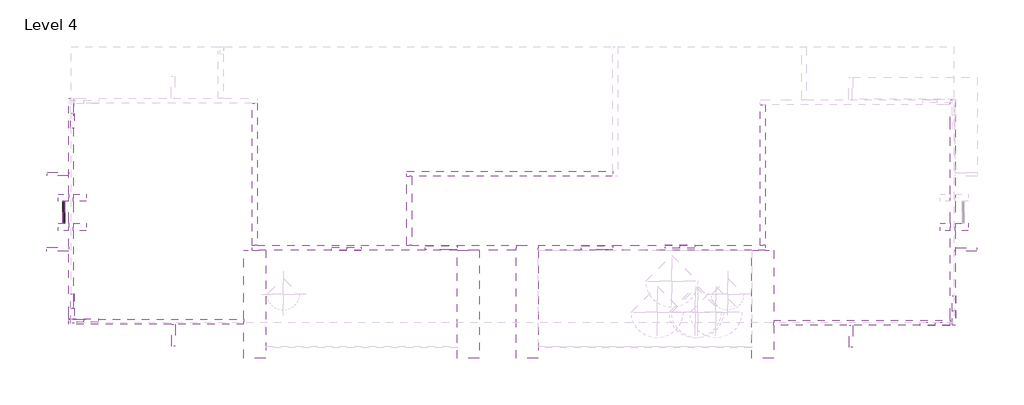
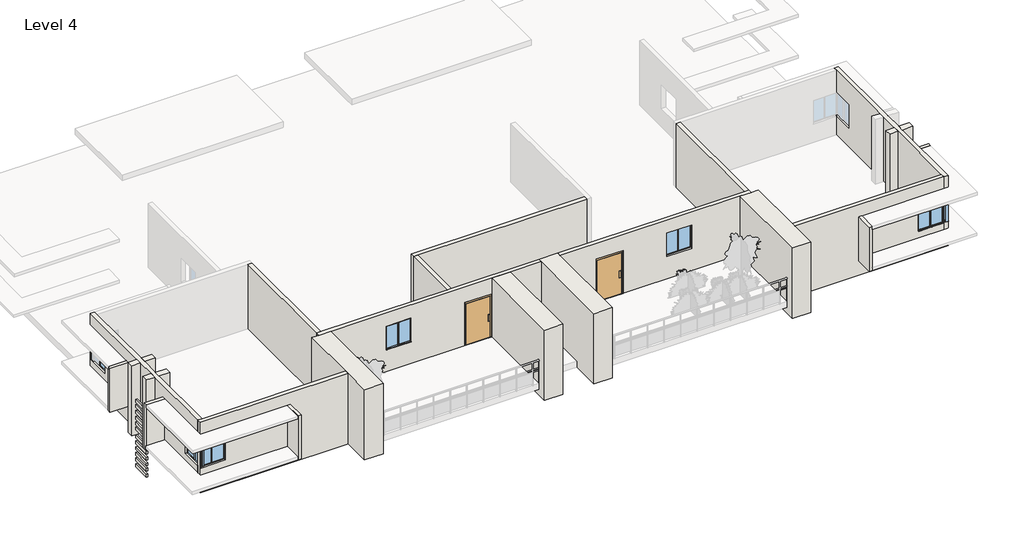
# One storey, part 1 of 4: 49 walls, 13 windows, 2 doors.
"""IFC4 building model written with IfcOpenShell, lengths in millimetres."""

from ifc_helpers import new_model, si_unit, frame, origin, place, context, project, spatial, polyline, outline, extrude, faceted_brep, transform, mapped, element, save
from components import door_15d3c954, window_20ff4747

model = new_model("IFC4")

# Units and contexts
model_context = context("Model", 3, world=origin())
ifc_project = project(units=[si_unit("LENGTHUNIT", "METRE", prefix="MILLI")], contexts=[model_context])

# Site, building, storey
site = spatial("IfcSite", under=ifc_project)
building = spatial("IfcBuilding", under=site)
storey = spatial("IfcBuildingStorey", under=building, Name="Level 4", Elevation=9144.0)

# Doors
placement = place(None, origin())
door_shape = door_15d3c954(model_context)
element("IfcDoor", 1, ObjectType="Door-Passage-Single-Flush-Dbl_Acting : 48\" x 96\"", at=placement, inside=storey, context=model_context, shape_type="MappedRepresentation", body=[
    mapped(door_shape, transform((7011.0520665, -5255.880811, 10972.8), x_axis=(-1.0, 0.0, 0.0), y_axis=(0.0, -1.0, 0.0), z_axis=(0.0, 0.0, 1.0))),
])
element("IfcDoor", 2, ObjectType="Door-Passage-Single-Flush-Dbl_Acting : 48\" x 96\"", at=placement, inside=storey, context=model_context, shape_type="MappedRepresentation", body=[
    mapped(door_shape, transform((559.4520665, -5255.1961695, 10972.8), x_axis=(-1.0, 0.0, 0.0), y_axis=(0.0, -1.0, 0.0), z_axis=(0.0, 0.0, 1.0))),
])

# Walls
element("IfcWall", 3, ObjectType="Generic - 1'", at=placement, inside=storey, context=model_context, shape_type="SweptSolid", body=[
    extrude(outline(polyline([(-14151.7972154, -3343.5294056), (-14680.5479335, -3343.5294056), (-14680.5479335, -3038.7294056), (-14151.7972154, -3038.7294056), (-14151.7972154, -3343.5294056)])), frame((0.0, 0.0, 10363.2), z_axis=(0.0, 0.0, 1.0), x_axis=(1.0, 0.0, 0.0)), (0.0, 0.0, 1.0), 3657.6),
])
element("IfcWall", 4, ObjectType="Generic - 1'", at=placement, inside=storey, context=model_context, shape_type="SweptSolid", body=[
    extrude(outline(polyline([(-15302.1394029, -3038.7294056), (-14883.7479335, -3038.7294056), (-14883.7479335, -3343.5294056), (-15302.1394029, -3343.5294056), (-15302.1394029, -3038.7294056)])), frame((0.0, 0.0, 10363.2), z_axis=(0.0, 0.0, 1.0), x_axis=(1.0, 0.0, 0.0)), (0.0, 0.0, 1.0), 3657.6),
])
element("IfcWall", 5, ObjectType="Generic - 1'", at=placement, inside=storey, context=model_context, shape_type="SweptSolid", body=[
    extrude(outline(polyline([(-14151.7972154, -4562.7294056), (-14680.5479335, -4562.7294056), (-14680.5479335, -4257.9294056), (-14151.7972154, -4257.9294056), (-14151.7972154, -4562.7294056)])), frame((0.0, 0.0, 10363.2), z_axis=(0.0, 0.0, 1.0), x_axis=(1.0, 0.0, 0.0)), (0.0, 0.0, 1.0), 3657.6),
])
element("IfcWall", 6, ObjectType="Generic - 1'", at=placement, inside=storey, context=model_context, shape_type="SweptSolid", body=[
    extrude(outline(polyline([(-15302.1394029, -4257.9294056), (-14883.7479335, -4257.9294056), (-14883.7479335, -4562.7294056), (-15302.1394029, -4562.7294056), (-15302.1394029, -4257.9294056)])), frame((0.0, 0.0, 10363.2), z_axis=(0.0, 0.0, 1.0), x_axis=(1.0, 0.0, 0.0)), (0.0, 0.0, 1.0), 3657.6),
])
element("IfcWall", 7, ObjectType="Generic - 1'", at=placement, inside=storey, context=model_context, shape_type="SweptSolid", body=[
    extrude(outline(polyline([(22386.1027846, -4562.7294056), (21857.3520665, -4562.7294056), (21857.3520665, -4257.9294056), (22386.1027846, -4257.9294056), (22386.1027846, -4562.7294056)])), frame((0.0, 0.0, 10363.2), z_axis=(0.0, 0.0, 1.0), x_axis=(1.0, 0.0, 0.0)), (0.0, 0.0, 1.0), 3657.6),
])
element("IfcWall", 8, ObjectType="Generic - 1'", at=placement, inside=storey, context=model_context, shape_type="SweptSolid", body=[
    extrude(outline(polyline([(21235.7605971, -4257.9294056), (21654.1520665, -4257.9294056), (21654.1520665, -4562.7294056), (21235.7605971, -4562.7294056), (21235.7605971, -4257.9294056)])), frame((0.0, 0.0, 10363.2), z_axis=(0.0, 0.0, 1.0), x_axis=(1.0, 0.0, 0.0)), (0.0, 0.0, 1.0), 3657.6),
])
element("IfcWall", 9, ObjectType="Generic - 3'", at=placement, inside=storey, context=model_context, shape_type="Brep", body=[
    faceted_brep([(2134.2520665, -9833.5461695, 10363.2), (2134.2520665, -5363.1461695, 10363.2), (2134.2520665, -5363.1461695, 14020.8), (2134.2520665, -9833.5461695, 14020.8), (1219.8520665, -9833.5461695, 10363.2), (1219.8520665, -9833.5461695, 14020.8), (1219.8520665, -5363.1461695, 14020.8), (1219.8520665, -5363.1461695, 13208.0), (1219.8520665, -5363.1461695, 10972.8), (1219.8520665, -5363.1461695, 10363.2)], [[[0, 1, 2, 3]], [[4, 5, 6, 7, 8, 9]], [[1, 0, 4, 9]], [[3, 2, 6, 5]], [[0, 3, 5, 4]], [[2, 1, 9, 8, 7, 6]]]),
])
element("IfcWall", 10, ObjectType="Generic - 3'", at=placement, inside=storey, context=model_context, shape_type="Brep", body=[
    faceted_brep([(4572.6520665, -9833.5461695, 10363.2), (4572.6520665, -5363.830811, 10363.2), (4572.6520665, -5160.630811, 10363.2), (4572.6520665, -5160.630811, 14020.8), (4572.6520665, -5363.830811, 14020.8), (4572.6520665, -9833.5461695, 14020.8), (3658.2520665, -9833.5461695, 10363.2), (3658.2520665, -9833.5461695, 14020.8), (3658.2520665, -5363.1461695, 14020.8), (3658.2520665, -5160.630811, 14020.8), (3658.2520665, -5160.630811, 10363.2), (3658.2520665, -5363.1461695, 10363.2)], [[[0, 1, 2, 3, 4, 5]], [[6, 7, 8, 9, 10, 11]], [[2, 1, 0, 6, 11, 10]], [[5, 4, 3, 9, 8, 7]], [[0, 5, 7, 6]], [[3, 2, 10, 9]]]),
])
element("IfcWall", 11, ObjectType="Generic - 3'", at=placement, inside=storey, context=model_context, shape_type="Brep", body=[
    faceted_brep([(-7619.3479335, -5363.1461695, 10363.2), (-7619.3479335, -8237.0604699, 10363.2), (-7619.3479335, -8440.2604699, 10363.2), (-7619.3479335, -9833.5461695, 10363.2), (-7619.3479335, -9833.5461695, 14020.8), (-7619.3479335, -8440.2604699, 14020.8), (-7619.3479335, -8237.0604699, 14020.8), (-7619.3479335, -5363.1461695, 14020.8), (-6704.9479335, -5363.1461695, 10363.2), (-6704.9479335, -5363.1461695, 14020.8), (-6704.9479335, -9833.5461695, 14020.8), (-6704.9479335, -9833.5461695, 10363.2), (-7263.7479335, -5363.1461695, 10363.2), (-7263.7479335, -5363.1461695, 14020.8)], [[[0, 1, 2, 3, 4, 5, 6, 7]], [[8, 9, 10, 11]], [[3, 2, 1, 0, 12, 8, 11]], [[4, 3, 11, 10]], [[7, 6, 5, 4, 10, 9, 13]], [[0, 7, 13, 9, 8, 12]]]),
])
element("IfcWall", 12, ObjectType="Generic - 3'", at=placement, inside=storey, context=model_context, shape_type="Brep", body=[
    faceted_brep([(13411.8520665, -5363.830811, 10363.2), (13411.8520665, -9834.230811, 10363.2), (13411.8520665, -9834.230811, 14020.8), (13411.8520665, -5363.830811, 14020.8), (14326.2520665, -5363.830811, 10363.2), (14326.2520665, -5363.830811, 14020.8), (14326.2520665, -8263.1451114, 14020.8), (14326.2520665, -8466.3451114, 14020.8), (14326.2520665, -9834.230811, 14020.8), (14326.2520665, -9834.230811, 10363.2), (14326.2520665, -8466.3451114, 10363.2), (14326.2520665, -8263.1451114, 10363.2), (13970.6520665, -5363.830811, 10363.2), (13970.6520665, -5363.830811, 14020.8)], [[[0, 1, 2, 3]], [[4, 5, 6, 7, 8, 9, 10, 11]], [[1, 0, 12, 4, 11, 10, 9]], [[2, 1, 9, 8]], [[3, 2, 8, 7, 6, 5, 13]], [[0, 3, 13, 5, 4, 12]]]),
])
element("IfcWall", 13, ObjectType="Generic - 5\"", at=placement, inside=storey, context=model_context, shape_type="SweptSolid", body=[
    extrude(outline(polyline([(-15124.6936682, -4257.9294056), (-15124.6936682, -3343.5294056), (-15048.4936682, -3343.5294056), (-15048.4936682, -4257.9294056), (-15124.6936682, -4257.9294056)])), frame((0.0, 0.0, 8712.2), z_axis=(0.0, 0.0, 1.0), x_axis=(1.0, 0.0, 0.0)), (0.0, 0.0, 1.0), 152.8735856),
])
element("IfcWall", 14, ObjectType="Generic - 5\"", at=placement, inside=storey, context=model_context, shape_type="SweptSolid", body=[
    extrude(outline(polyline([(-15124.6936682, -4257.9294056), (-15124.6936682, -3343.5294056), (-15048.4936682, -3343.5294056), (-15048.4936682, -4257.9294056), (-15124.6936682, -4257.9294056)])), frame((0.0, 0.0, 9017.0), z_axis=(0.0, 0.0, 1.0), x_axis=(1.0, 0.0, 0.0)), (0.0, 0.0, 1.0), 152.8735856),
])
element("IfcWall", 15, ObjectType="Generic - 5\"", at=placement, inside=storey, context=model_context, shape_type="SweptSolid", body=[
    extrude(outline(polyline([(-15124.6936682, -4257.9294056), (-15124.6936682, -3343.5294056), (-15048.4936682, -3343.5294056), (-15048.4936682, -4257.9294056), (-15124.6936682, -4257.9294056)])), frame((0.0, 0.0, 9296.4), z_axis=(0.0, 0.0, 1.0), x_axis=(1.0, 0.0, 0.0)), (0.0, 0.0, 1.0), 152.8735856),
])
element("IfcWall", 16, ObjectType="Generic - 5\"", at=placement, inside=storey, context=model_context, shape_type="SweptSolid", body=[
    extrude(outline(polyline([(-15124.6936682, -4257.9294056), (-15124.6936682, -3343.5294056), (-15048.4936682, -3343.5294056), (-15048.4936682, -4257.9294056), (-15124.6936682, -4257.9294056)])), frame((0.0, 0.0, 9601.2), z_axis=(0.0, 0.0, 1.0), x_axis=(1.0, 0.0, 0.0)), (0.0, 0.0, 1.0), 152.8735856),
])
element("IfcWall", 17, ObjectType="Generic - 5\"", at=placement, inside=storey, context=model_context, shape_type="SweptSolid", body=[
    extrude(outline(polyline([(-15124.6936682, -4257.9294056), (-15124.6936682, -3343.5294056), (-15048.4936682, -3343.5294056), (-15048.4936682, -4257.9294056), (-15124.6936682, -4257.9294056)])), frame((0.0, 0.0, 9906.0), z_axis=(0.0, 0.0, 1.0), x_axis=(1.0, 0.0, 0.0)), (0.0, 0.0, 1.0), 152.8735856),
])
element("IfcWall", 18, ObjectType="Generic - 5\"", at=placement, inside=storey, context=model_context, shape_type="SweptSolid", body=[
    extrude(outline(polyline([(-15124.6936682, -4257.9294056), (-15124.6936682, -3343.5294056), (-15048.4936682, -3343.5294056), (-15048.4936682, -4257.9294056), (-15124.6936682, -4257.9294056)])), frame((0.0, 0.0, 10210.8), z_axis=(0.0, 0.0, 1.0), x_axis=(1.0, 0.0, 0.0)), (0.0, 0.0, 1.0), 152.8735856),
])
element("IfcWall", 19, ObjectType="Generic - 5\"", at=placement, inside=storey, context=model_context, shape_type="SweptSolid", body=[
    extrude(outline(polyline([(-15124.6936682, -4257.9294056), (-15124.6936682, -3343.5294056), (-15048.4936682, -3343.5294056), (-15048.4936682, -4257.9294056), (-15124.6936682, -4257.9294056)])), frame((0.0, 0.0, 8712.2), z_axis=(0.0, 0.0, 1.0), x_axis=(1.0, 0.0, 0.0)), (0.0, 0.0, 1.0), 152.8735856),
])
element("IfcWall", 20, ObjectType="Generic - 5\"", at=placement, inside=storey, context=model_context, shape_type="SweptSolid", body=[
    extrude(outline(polyline([(-15124.6936682, -4257.9294056), (-15124.6936682, -3343.5294056), (-15048.4936682, -3343.5294056), (-15048.4936682, -4257.9294056), (-15124.6936682, -4257.9294056)])), frame((0.0, 0.0, 9017.0), z_axis=(0.0, 0.0, 1.0), x_axis=(1.0, 0.0, 0.0)), (0.0, 0.0, 1.0), 152.8735856),
])
element("IfcWall", 21, ObjectType="Generic - 5\"", at=placement, inside=storey, context=model_context, shape_type="SweptSolid", body=[
    extrude(outline(polyline([(-15124.6936682, -4257.9294056), (-15124.6936682, -3343.5294056), (-15048.4936682, -3343.5294056), (-15048.4936682, -4257.9294056), (-15124.6936682, -4257.9294056)])), frame((0.0, 0.0, 9296.4), z_axis=(0.0, 0.0, 1.0), x_axis=(1.0, 0.0, 0.0)), (0.0, 0.0, 1.0), 152.8735856),
])
element("IfcWall", 22, ObjectType="Generic - 5\"", at=placement, inside=storey, context=model_context, shape_type="SweptSolid", body=[
    extrude(outline(polyline([(-15124.6936682, -4257.9294056), (-15124.6936682, -3343.5294056), (-15048.4936682, -3343.5294056), (-15048.4936682, -4257.9294056), (-15124.6936682, -4257.9294056)])), frame((0.0, 0.0, 9601.2), z_axis=(0.0, 0.0, 1.0), x_axis=(1.0, 0.0, 0.0)), (0.0, 0.0, 1.0), 152.8735856),
])
element("IfcWall", 23, ObjectType="Generic - 5\"", at=placement, inside=storey, context=model_context, shape_type="SweptSolid", body=[
    extrude(outline(polyline([(-15124.6936682, -4257.9294056), (-15124.6936682, -3343.5294056), (-15048.4936682, -3343.5294056), (-15048.4936682, -4257.9294056), (-15124.6936682, -4257.9294056)])), frame((0.0, 0.0, 9906.0), z_axis=(0.0, 0.0, 1.0), x_axis=(1.0, 0.0, 0.0)), (0.0, 0.0, 1.0), 152.8735856),
])
element("IfcWall", 24, ObjectType="Generic - 5\"", at=placement, inside=storey, context=model_context, shape_type="SweptSolid", body=[
    extrude(outline(polyline([(-15124.6936682, -4257.9294056), (-15124.6936682, -3343.5294056), (-15048.4936682, -3343.5294056), (-15048.4936682, -4257.9294056), (-15124.6936682, -4257.9294056)])), frame((0.0, 0.0, 10210.8), z_axis=(0.0, 0.0, 1.0), x_axis=(1.0, 0.0, 0.0)), (0.0, 0.0, 1.0), 152.8735856),
])
element("IfcWall", 25, ObjectType="Generic - 5\"", at=placement, inside=storey, context=model_context, shape_type="SweptSolid", body=[
    extrude(outline(polyline([(-15124.6936682, -4257.9294056), (-15124.6936682, -3343.5294056), (-15048.4936682, -3343.5294056), (-15048.4936682, -4257.9294056), (-15124.6936682, -4257.9294056)])), frame((0.0, 0.0, 10617.2), z_axis=(0.0, 0.0, 1.0), x_axis=(1.0, 0.0, 0.0)), (0.0, 0.0, 1.0), 152.8735856),
])
element("IfcWall", 26, ObjectType="Generic - 5\"", at=placement, inside=storey, context=model_context, shape_type="SweptSolid", body=[
    extrude(outline(polyline([(-15124.6936682, -4257.9294056), (-15124.6936682, -3343.5294056), (-15048.4936682, -3343.5294056), (-15048.4936682, -4257.9294056), (-15124.6936682, -4257.9294056)])), frame((0.0, 0.0, 10896.6), z_axis=(0.0, 0.0, 1.0), x_axis=(1.0, 0.0, 0.0)), (0.0, 0.0, 1.0), 152.8735856),
])
element("IfcWall", 27, ObjectType="Generic - 5\"", at=placement, inside=storey, context=model_context, shape_type="SweptSolid", body=[
    extrude(outline(polyline([(-15124.6936682, -4257.9294056), (-15124.6936682, -3343.5294056), (-15048.4936682, -3343.5294056), (-15048.4936682, -4257.9294056), (-15124.6936682, -4257.9294056)])), frame((0.0, 0.0, 11176.0), z_axis=(0.0, 0.0, 1.0), x_axis=(1.0, 0.0, 0.0)), (0.0, 0.0, 1.0), 152.8735856),
])
element("IfcWall", 28, ObjectType="Generic - 5\"", at=placement, inside=storey, context=model_context, shape_type="SweptSolid", body=[
    extrude(outline(polyline([(-15124.6936682, -4257.9294056), (-15124.6936682, -3343.5294056), (-15048.4936682, -3343.5294056), (-15048.4936682, -4257.9294056), (-15124.6936682, -4257.9294056)])), frame((0.0, 0.0, 11480.8), z_axis=(0.0, 0.0, 1.0), x_axis=(1.0, 0.0, 0.0)), (0.0, 0.0, 1.0), 152.8735856),
])
element("IfcWall", 29, ObjectType="Generic - 5\"", at=placement, inside=storey, context=model_context, shape_type="SweptSolid", body=[
    extrude(outline(polyline([(-15124.6936682, -4257.9294056), (-15124.6936682, -3343.5294056), (-15048.4936682, -3343.5294056), (-15048.4936682, -4257.9294056), (-15124.6936682, -4257.9294056)])), frame((0.0, 0.0, 11785.6), z_axis=(0.0, 0.0, 1.0), x_axis=(1.0, 0.0, 0.0)), (0.0, 0.0, 1.0), 152.8735856),
])
element("IfcWall", 30, ObjectType="Generic - 5\"", at=placement, inside=storey, context=model_context, shape_type="SweptSolid", body=[
    extrude(outline(polyline([(-15124.6936682, -4257.9294056), (-15124.6936682, -3343.5294056), (-15048.4936682, -3343.5294056), (-15048.4936682, -4257.9294056), (-15124.6936682, -4257.9294056)])), frame((0.0, 0.0, 12065.0), z_axis=(0.0, 0.0, 1.0), x_axis=(1.0, 0.0, 0.0)), (0.0, 0.0, 1.0), 152.8735856),
])
element("IfcWall", 31, ObjectType="Generic - 5\"", at=placement, inside=storey, context=model_context, shape_type="SweptSolid", body=[
    extrude(outline(polyline([(-15124.6936682, -4257.9294056), (-15124.6936682, -3343.5294056), (-15048.4936682, -3343.5294056), (-15048.4936682, -4257.9294056), (-15124.6936682, -4257.9294056)])), frame((0.0, 0.0, 10617.2), z_axis=(0.0, 0.0, 1.0), x_axis=(1.0, 0.0, 0.0)), (0.0, 0.0, 1.0), 152.8735856),
])
element("IfcWall", 32, ObjectType="Generic - 5\"", at=placement, inside=storey, context=model_context, shape_type="SweptSolid", body=[
    extrude(outline(polyline([(-15124.6936682, -4257.9294056), (-15124.6936682, -3343.5294056), (-15048.4936682, -3343.5294056), (-15048.4936682, -4257.9294056), (-15124.6936682, -4257.9294056)])), frame((0.0, 0.0, 10896.6), z_axis=(0.0, 0.0, 1.0), x_axis=(1.0, 0.0, 0.0)), (0.0, 0.0, 1.0), 152.8735856),
])
element("IfcWall", 33, ObjectType="Generic - 5\"", at=placement, inside=storey, context=model_context, shape_type="SweptSolid", body=[
    extrude(outline(polyline([(-15124.6936682, -4257.9294056), (-15124.6936682, -3343.5294056), (-15048.4936682, -3343.5294056), (-15048.4936682, -4257.9294056), (-15124.6936682, -4257.9294056)])), frame((0.0, 0.0, 11176.0), z_axis=(0.0, 0.0, 1.0), x_axis=(1.0, 0.0, 0.0)), (0.0, 0.0, 1.0), 152.8735856),
])
element("IfcWall", 34, ObjectType="Generic - 5\"", at=placement, inside=storey, context=model_context, shape_type="SweptSolid", body=[
    extrude(outline(polyline([(-15124.6936682, -4257.9294056), (-15124.6936682, -3343.5294056), (-15048.4936682, -3343.5294056), (-15048.4936682, -4257.9294056), (-15124.6936682, -4257.9294056)])), frame((0.0, 0.0, 11480.8), z_axis=(0.0, 0.0, 1.0), x_axis=(1.0, 0.0, 0.0)), (0.0, 0.0, 1.0), 152.8735856),
])
element("IfcWall", 35, ObjectType="Generic - 5\"", at=placement, inside=storey, context=model_context, shape_type="SweptSolid", body=[
    extrude(outline(polyline([(-15124.6936682, -4257.9294056), (-15124.6936682, -3343.5294056), (-15048.4936682, -3343.5294056), (-15048.4936682, -4257.9294056), (-15124.6936682, -4257.9294056)])), frame((0.0, 0.0, 11785.6), z_axis=(0.0, 0.0, 1.0), x_axis=(1.0, 0.0, 0.0)), (0.0, 0.0, 1.0), 152.8735856),
])
element("IfcWall", 36, ObjectType="Generic - 5\"", at=placement, inside=storey, context=model_context, shape_type="SweptSolid", body=[
    extrude(outline(polyline([(-15124.6936682, -4257.9294056), (-15124.6936682, -3343.5294056), (-15048.4936682, -3343.5294056), (-15048.4936682, -4257.9294056), (-15124.6936682, -4257.9294056)])), frame((0.0, 0.0, 12065.0), z_axis=(0.0, 0.0, 1.0), x_axis=(1.0, 0.0, 0.0)), (0.0, 0.0, 1.0), 152.8735856),
])
element("IfcWall", 37, ObjectType="Generic - 6\"", at=placement, inside=storey, context=model_context, shape_type="SweptSolid", body=[
    extrude(outline(polyline([(22749.4138484, -5418.3451114), (21857.3520665, -5418.3451114), (21857.3520665, -5265.9451114), (22749.4138484, -5265.9451114), (22749.4138484, -5418.3451114)])), frame((0.0, 0.0, 11125.2), z_axis=(0.0, 0.0, 1.0), x_axis=(1.0, 0.0, 0.0)), (0.0, 0.0, 1.0), 2286.0),
])
element("IfcWall", 38, ObjectType="Generic - 6\"", at=placement, inside=storey, context=model_context, shape_type="SweptSolid", body=[
    extrude(outline(polyline([(17454.3075984, -9380.7451114), (17454.3075984, -8466.3451114), (17606.7075984, -8466.3451114), (17606.7075984, -9380.7451114), (17454.3075984, -9380.7451114)])), frame((0.0, 0.0, 11125.2), z_axis=(0.0, 0.0, 1.0), x_axis=(1.0, 0.0, 0.0)), (0.0, 0.0, 1.0), 2286.0),
])
element("IfcWall", 39, ObjectType="Generic - 6\"", at=placement, inside=storey, context=model_context, shape_type="SweptSolid", body=[
    extrude(outline(polyline([(-15775.8097154, -2128.3604699), (-14883.7479335, -2128.3604699), (-14883.7479335, -2280.7604699), (-15775.8097154, -2280.7604699), (-15775.8097154, -2128.3604699)])), frame((0.0, 0.0, 11125.2), z_axis=(0.0, 0.0, 1.0), x_axis=(1.0, 0.0, 0.0)), (0.0, 0.0, 1.0), 2286.0),
])
element("IfcWall", 40, ObjectType="Generic - 6\"", at=placement, inside=storey, context=model_context, shape_type="SweptSolid", body=[
    extrude(outline(polyline([(-15796.5604335, -5250.9729699), (-14883.7479335, -5250.9729699), (-14883.7479335, -5403.3729699), (-15796.5604335, -5403.3729699), (-15796.5604335, -5250.9729699)])), frame((0.0, 0.0, 11125.2), z_axis=(0.0, 0.0, 1.0), x_axis=(1.0, 0.0, 0.0)), (0.0, 0.0, 1.0), 2286.0),
])
element("IfcWall", 41, ObjectType="Generic - 6\"", at=placement, inside=storey, context=model_context, shape_type="SweptSolid", body=[
    extrude(outline(polyline([(-10607.7034654, -9354.6604699), (-10607.7034654, -8440.2604699), (-10455.3034654, -8440.2604699), (-10455.3034654, -9354.6604699), (-10607.7034654, -9354.6604699)])), frame((0.0, 0.0, 11125.2), z_axis=(0.0, 0.0, 1.0), x_axis=(1.0, 0.0, 0.0)), (0.0, 0.0, 1.0), 2286.0),
])
element("IfcWall", 42, ObjectType="Generic - 8\"", at=placement, inside=storey, context=model_context, shape_type="Brep", body=[
    faceted_brep([(7671.4520665, -2102.9604699, 10972.8), (-862.9479335, -2102.9604699, 10972.8), (-862.9479335, -2102.9604699, 14020.8), (7671.4520665, -2102.9604699, 14020.8), (7671.4520665, -2306.1604699, 10972.8), (7671.4520665, -2306.1604699, 14020.8), (-659.7479335, -2306.1604699, 14020.8), (-862.9479335, -2306.1604699, 14020.8), (-862.9479335, -2306.1604699, 10972.8), (-659.7479335, -2306.1604699, 10972.8)], [[[0, 1, 2, 3]], [[4, 5, 6, 7, 8, 9]], [[1, 0, 4, 9, 8]], [[3, 2, 7, 6, 5]], [[0, 3, 5, 4]], [[2, 1, 8, 7]]]),
])
element("IfcWall", 43, ObjectType="Generic - 8\"", at=placement, inside=storey, context=model_context, shape_type="SweptSolid", body=[
    extrude(outline(polyline([(-862.9479335, -5159.9461695), (-862.9479335, -2306.1604699), (-659.7479335, -2306.1604699), (-659.7479335, -5159.9461695), (-862.9479335, -5159.9461695)])), frame((0.0, 0.0, 10972.8), z_axis=(0.0, 0.0, 1.0), x_axis=(1.0, 0.0, 0.0)), (0.0, 0.0, 1.0), 3048.0),
])
element("IfcWall", 44, ObjectType="Generic - 8\" gray", at=placement, inside=storey, context=model_context, shape_type="Brep", body=[
    faceted_brep([(-14883.7479335, -8440.2604699, 10363.2), (-7619.3479335, -8440.2604699, 10363.2), (-7619.3479335, -8440.2604699, 14020.8), (-14883.7479335, -8440.2604699, 14020.8), (-13655.3509584, -8440.2604699, 11635.4804451), (-14874.5509584, -8440.2604699, 11635.4804451), (-14874.5509584, -8440.2604699, 12854.6804451), (-13655.3509584, -8440.2604699, 12854.6804451), (-7619.3479335, -8237.0604699, 10363.2), (-14680.5479335, -8237.0604699, 10363.2), (-14883.7479335, -8237.0604699, 10363.2), (-14883.7479335, -8237.0604699, 11635.4804451), (-14883.7479335, -8237.0604699, 12854.6804451), (-14883.7479335, -8237.0604699, 14020.8), (-14680.5479335, -8237.0604699, 14020.8), (-7619.3479335, -8237.0604699, 14020.8), (-14874.5509584, -8237.0604699, 11635.4804451), (-14680.5479335, -8237.0604699, 11635.4804451), (-13655.3509584, -8237.0604699, 11635.4804451), (-13655.3509584, -8237.0604699, 12854.6804451), (-14680.5479335, -8237.0604699, 12854.6804451), (-14874.5509584, -8237.0604699, 12854.6804451)], [[[0, 1, 2, 3], [4, 5, 6, 7]], [[8, 9, 10, 11, 12, 13, 14, 15], [16, 17, 18, 19, 20, 21]], [[1, 0, 10, 9, 8]], [[3, 2, 15, 14, 13]], [[0, 3, 13, 12, 11, 10]], [[2, 1, 8, 15]], [[4, 18, 17, 16, 5]], [[6, 5, 16, 21]], [[6, 21, 20, 19, 7]], [[7, 19, 18, 4]]]),
])
element("IfcWall", 45, ObjectType="Generic - 8\" gray", at=placement, inside=storey, context=model_context, shape_type="Brep", body=[
    faceted_brep([(-14883.7479335, 919.6395301, 10363.2), (-14883.7479335, -3038.7294056, 10363.2), (-14883.7479335, -3343.5294056, 10363.2), (-14883.7479335, -4257.9294056, 10363.2), (-14883.7479335, -4562.7294056, 10363.2), (-14883.7479335, -8237.0604699, 10363.2), (-14883.7479335, -8237.0604699, 11635.4804451), (-14883.7479335, -7169.263768, 11635.4804451), (-14883.7479335, -7169.263768, 12854.6804451), (-14883.7479335, -8237.0604699, 12854.6804451), (-14883.7479335, -8237.0604699, 14020.8), (-14883.7479335, -4562.7294056, 14020.8), (-14883.7479335, -4257.9294056, 14020.8), (-14883.7479335, -3343.5294056, 14020.8), (-14883.7479335, -3038.7294056, 14020.8), (-14883.7479335, 919.6395301, 14020.8), (-14883.7479335, -310.2864811, 11635.4804451), (-14883.7479335, 908.9135189, 11635.4804451), (-14883.7479335, 908.9135189, 12854.6804451), (-14883.7479335, -310.2864811, 12854.6804451), (-14680.5479335, -8237.0604699, 10363.2), (-14680.5479335, -4562.7294056, 10363.2), (-14680.5479335, -4257.9294056, 10363.2), (-14680.5479335, -3343.5294056, 10363.2), (-14680.5479335, -3038.7294056, 10363.2), (-14680.5479335, 716.4395301, 10363.2), (-14680.5479335, 919.6395301, 10363.2), (-14680.5479335, 919.6395301, 11635.4804451), (-14680.5479335, 919.6395301, 12854.6804451), (-14680.5479335, 919.6395301, 14020.8), (-14680.5479335, 716.4395301, 14020.8), (-14680.5479335, -3038.7294056, 14020.8), (-14680.5479335, -3343.5294056, 14020.8), (-14680.5479335, -4257.9294056, 14020.8), (-14680.5479335, -4562.7294056, 14020.8), (-14680.5479335, -8237.0604699, 14020.8), (-14680.5479335, -8237.0604699, 12854.6804451), (-14680.5479335, -7169.263768, 12854.6804451), (-14680.5479335, -7169.263768, 11635.4804451), (-14680.5479335, -8237.0604699, 11635.4804451), (-14680.5479335, 908.9135189, 11635.4804451), (-14680.5479335, 716.4395301, 11635.4804451), (-14680.5479335, -310.2864811, 11635.4804451), (-14680.5479335, -310.2864811, 12854.6804451), (-14680.5479335, 716.4395301, 12854.6804451), (-14680.5479335, 908.9135189, 12854.6804451), (-14874.5509584, -8237.0604699, 11635.4804451), (-14874.5509584, -8237.0604699, 12854.6804451)], [[[0, 1, 2, 3, 4, 5, 6, 7, 8, 9, 10, 11, 12, 13, 14, 15], [16, 17, 18, 19]], [[20, 21, 22, 23, 24, 25, 26, 27, 28, 29, 30, 31, 32, 33, 34, 35, 36, 37, 38, 39], [40, 41, 42, 43, 44, 45]], [[5, 4, 3, 2, 1, 0, 26, 25, 24, 23, 22, 21, 20]], [[15, 14, 13, 12, 11, 10, 35, 34, 33, 32, 31, 30, 29]], [[0, 15, 29, 28, 27, 26]], [[5, 20, 39, 46, 6]], [[35, 10, 9, 47, 36]], [[38, 7, 6, 46, 39]], [[8, 7, 38, 37]], [[8, 37, 36, 47, 9]], [[16, 42, 41, 40, 17]], [[18, 45, 44, 43, 19]], [[19, 43, 42, 16]], [[45, 18, 17, 40]]]),
])
element("IfcWall", 46, ObjectType="Generic - 8\" gray", at=placement, inside=storey, context=model_context, shape_type="Brep", body=[
    faceted_brep([(21654.1520665, 868.1548886, 10363.2), (21654.1520665, 664.9548886, 10363.2), (21654.1520665, -3038.7294056, 10363.2), (21654.1520665, -3343.5294056, 10363.2), (21654.1520665, -4257.9294056, 10363.2), (21654.1520665, -4562.7294056, 10363.2), (21654.1520665, -8263.1451114, 10363.2), (21654.1520665, -8466.3451114, 10363.2), (21654.1520665, -8466.3451114, 11635.4804451), (21654.1520665, -7262.9130582, 11635.4804451), (21654.1520665, -7262.9130582, 12854.6804451), (21654.1520665, -8466.3451114, 12854.6804451), (21654.1520665, -8466.3451114, 14020.8), (21654.1520665, -8263.1451114, 14020.8), (21654.1520665, -4562.7294056, 14020.8), (21654.1520665, -4257.9294056, 14020.8), (21654.1520665, -3343.5294056, 14020.8), (21654.1520665, -3038.7294056, 14020.8), (21654.1520665, 664.9548886, 14020.8), (21654.1520665, 868.1548886, 14020.8), (21654.1520665, 868.1548886, 12854.6804451), (21654.1520665, 868.1548886, 11635.4804451), (21654.1520665, 859.364485, 11635.4804451), (21654.1520665, 859.364485, 12854.6804451), (21654.1520665, 664.9548886, 12854.6804451), (21654.1520665, -359.835515, 12854.6804451), (21654.1520665, -359.835515, 11635.4804451), (21654.1520665, 664.9548886, 11635.4804451), (21857.3520665, -8466.3451114, 10363.2), (21857.3520665, -4562.7294056, 10363.2), (21857.3520665, -4257.9294056, 10363.2), (21857.3520665, -3343.5294056, 10363.2), (21857.3520665, -3038.7294056, 10363.2), (21857.3520665, 868.1548886, 10363.2), (21857.3520665, 868.1548886, 14020.8), (21857.3520665, -3038.7294056, 14020.8), (21857.3520665, -3343.5294056, 14020.8), (21857.3520665, -4257.9294056, 14020.8), (21857.3520665, -4562.7294056, 14020.8), (21857.3520665, -8466.3451114, 14020.8), (21857.3520665, -8466.3451114, 12854.6804451), (21857.3520665, -7262.9130582, 12854.6804451), (21857.3520665, -7262.9130582, 11635.4804451), (21857.3520665, -8466.3451114, 11635.4804451), (21857.3520665, 859.364485, 12854.6804451), (21857.3520665, 859.364485, 11635.4804451), (21857.3520665, -359.835515, 11635.4804451), (21857.3520665, -359.835515, 12854.6804451)], [[[0, 1, 2, 3, 4, 5, 6, 7, 8, 9, 10, 11, 12, 13, 14, 15, 16, 17, 18, 19, 20, 21], [22, 23, 24, 25, 26, 27]], [[28, 29, 30, 31, 32, 33, 34, 35, 36, 37, 38, 39, 40, 41, 42, 43], [44, 45, 46, 47]], [[7, 6, 5, 4, 3, 2, 1, 0, 33, 32, 31, 30, 29, 28]], [[19, 18, 17, 16, 15, 14, 13, 12, 39, 38, 37, 36, 35, 34]], [[0, 21, 20, 19, 34, 33]], [[7, 28, 43, 8]], [[39, 12, 11, 40]], [[45, 22, 27, 26, 46]], [[23, 22, 45, 44]], [[23, 44, 47, 25, 24]], [[25, 47, 46, 26]], [[8, 43, 42, 9]], [[10, 9, 42, 41]], [[10, 41, 40, 11]]]),
])
element("IfcWall", 47, ObjectType="Generic - 8\" gray", at=placement, inside=storey, context=model_context, shape_type="Brep", body=[
    faceted_brep([(3658.2520665, -5159.9461695, 10363.2), (-7060.5479335, -5159.9461695, 10363.2), (-7263.7479335, -5159.9461695, 10363.2), (-7263.7479335, -5159.9461695, 14020.8), (-7060.5479335, -5159.9461695, 14020.8), (-862.9479335, -5159.9461695, 14020.8), (-659.7479335, -5159.9461695, 14020.8), (3658.2520665, -5159.9461695, 14020.8), (-2753.0651847, -5159.9461695, 12112.2951112), (-2753.0651847, -5159.9461695, 13331.4951112), (-3972.2651847, -5159.9461695, 13331.4951112), (-3972.2651847, -5159.9461695, 12112.2951112), (-100.9479335, -5159.9461695, 13208.0), (-100.9479335, -5159.9461695, 10972.8), (1219.8520665, -5159.9461695, 10972.8), (1219.8520665, -5159.9461695, 13208.0), (-7263.7479335, -5363.1461695, 10363.2), (-6704.9479335, -5363.1461695, 10363.2), (1219.8520665, -5363.1461695, 10363.2), (2134.2520665, -5363.1461695, 10363.2), (3658.2520665, -5363.1461695, 10363.2), (3658.2520665, -5363.1461695, 14020.8), (2134.2520665, -5363.1461695, 14020.8), (1219.8520665, -5363.1461695, 14020.8), (-6704.9479335, -5363.1461695, 14020.8), (-7263.7479335, -5363.1461695, 14020.8), (-2753.0651847, -5363.1461695, 13331.4951112), (-2753.0651847, -5363.1461695, 12112.2951112), (-3972.2651847, -5363.1461695, 12112.2951112), (-3972.2651847, -5363.1461695, 13331.4951112), (-100.9479335, -5363.1461695, 10972.8), (-100.9479335, -5363.1461695, 13208.0), (1219.8520665, -5363.1461695, 13208.0), (1219.8520665, -5363.1461695, 10972.8), (3658.2520665, -5160.630811, 10363.2), (3658.2520665, -5160.630811, 14020.8)], [[[0, 1, 2, 3, 4, 5, 6, 7], [8, 9, 10, 11], [12, 13, 14, 15]], [[16, 17, 18, 19, 20, 21, 22, 23, 24, 25], [26, 27, 28, 29], [30, 31, 32, 33]], [[2, 1, 0, 34, 20, 19, 18, 17, 16]], [[7, 6, 5, 4, 3, 25, 24, 23, 22, 21, 35]], [[0, 7, 35, 21, 20, 34]], [[3, 2, 16, 25]], [[27, 8, 11, 28]], [[9, 8, 27, 26]], [[9, 26, 29, 10]], [[10, 29, 28, 11]], [[30, 13, 12, 31]], [[31, 12, 15, 32]], [[32, 15, 14, 33]], [[13, 30, 33, 14]]]),
])
element("IfcWall", 48, ObjectType="Generic - 8\" gray", at=placement, inside=storey, context=model_context, shape_type="Brep", body=[
    faceted_brep([(4572.6520665, -5363.830811, 10363.2), (13411.8520665, -5363.830811, 10363.2), (13970.6520665, -5363.830811, 10363.2), (13970.6520665, -5363.830811, 14020.8), (13411.8520665, -5363.830811, 14020.8), (4572.6520665, -5363.830811, 14020.8), (9831.9980014, -5363.830811, 12131.0493508), (9831.9980014, -5363.830811, 13350.2493508), (11051.1980014, -5363.830811, 13350.2493508), (11051.1980014, -5363.830811, 12131.0493508), (6350.6520665, -5363.830811, 10972.8), (6350.6520665, -5363.830811, 13208.0), (7671.4520665, -5363.830811, 13208.0), (7671.4520665, -5363.830811, 10972.8), (13970.6520665, -5160.630811, 10363.2), (13767.4520665, -5160.630811, 10363.2), (4572.6520665, -5160.630811, 10363.2), (4572.6520665, -5160.630811, 14020.8), (13767.4520665, -5160.630811, 14020.8), (13970.6520665, -5160.630811, 14020.8), (9831.9980014, -5160.630811, 13350.2493508), (9831.9980014, -5160.630811, 12131.0493508), (11051.1980014, -5160.630811, 12131.0493508), (11051.1980014, -5160.630811, 13350.2493508), (6350.6520665, -5160.630811, 13208.0), (6350.6520665, -5160.630811, 10972.8), (7671.4520665, -5160.630811, 10972.8), (7671.4520665, -5160.630811, 13208.0)], [[[0, 1, 2, 3, 4, 5], [6, 7, 8, 9], [10, 11, 12, 13]], [[14, 15, 16, 17, 18, 19], [20, 21, 22, 23], [24, 25, 26, 27]], [[2, 1, 0, 16, 15, 14]], [[5, 4, 3, 19, 18, 17]], [[0, 5, 17, 16]], [[3, 2, 14, 19]], [[21, 6, 9, 22]], [[7, 6, 21, 20]], [[7, 20, 23, 8]], [[8, 23, 22, 9]], [[10, 25, 24, 11]], [[11, 24, 27, 12]], [[12, 27, 26, 13]], [[25, 10, 13, 26]]]),
])
element("IfcWall", 49, ObjectType="Generic - 8\" gray", at=placement, inside=storey, context=model_context, shape_type="Brep", body=[
    faceted_brep([(21654.1520665, -8263.1451114, 10363.2), (14326.2520665, -8263.1451114, 10363.2), (14326.2520665, -8263.1451114, 14020.8), (21654.1520665, -8263.1451114, 14020.8), (20403.2295783, -8263.1451114, 11635.4804451), (21622.4295783, -8263.1451114, 11635.4804451), (21622.4295783, -8263.1451114, 12854.6804451), (20403.2295783, -8263.1451114, 12854.6804451), (14326.2520665, -8466.3451114, 10363.2), (21654.1520665, -8466.3451114, 10363.2), (21654.1520665, -8466.3451114, 11635.4804451), (21654.1520665, -8466.3451114, 12854.6804451), (21654.1520665, -8466.3451114, 14020.8), (14326.2520665, -8466.3451114, 14020.8), (21622.4295783, -8466.3451114, 11635.4804451), (20403.2295783, -8466.3451114, 11635.4804451), (20403.2295783, -8466.3451114, 12854.6804451), (21622.4295783, -8466.3451114, 12854.6804451)], [[[0, 1, 2, 3], [4, 5, 6, 7]], [[8, 9, 10, 11, 12, 13], [14, 15, 16, 17]], [[1, 0, 9, 8]], [[3, 2, 13, 12]], [[0, 3, 12, 11, 10, 9]], [[2, 1, 8, 13]], [[4, 15, 14, 5]], [[6, 5, 14, 17]], [[6, 17, 16, 7]], [[7, 16, 15, 4]]]),
])
element("IfcWall", 50, ObjectType="Generic - 8\" gray", at=placement, inside=storey, context=model_context, shape_type="SweptSolid", body=[
    extrude(outline(polyline([(-7263.7479335, -5159.9461695), (-7263.7479335, 716.4395301), (-7060.5479335, 716.4395301), (-7060.5479335, -5159.9461695), (-7263.7479335, -5159.9461695)])), frame((0.0, 0.0, 10363.2), z_axis=(0.0, 0.0, 1.0), x_axis=(1.0, 0.0, 0.0)), (0.0, 0.0, 1.0), 3657.6),
])
element("IfcWall", 51, ObjectType="Generic - 8\" gray", at=placement, inside=storey, context=model_context, shape_type="SweptSolid", body=[
    extrude(outline(polyline([(13767.4520665, -5160.630811), (13767.4520665, 664.9548886), (13970.6520665, 664.9548886), (13970.6520665, -5160.630811), (13767.4520665, -5160.630811)])), frame((0.0, 0.0, 10363.2), z_axis=(0.0, 0.0, 1.0), x_axis=(1.0, 0.0, 0.0)), (0.0, 0.0, 1.0), 3657.6),
])

# Windows
window_shape = window_20ff4747(model_context)
element("IfcWindow", 52, ObjectType="Instance - Fixed : 24\" x 48\"", at=placement, inside=storey, context=model_context, shape_type="MappedRepresentation", body=[
    mapped(window_shape, transform((21755.7520665, -8215.4130582, 10721.0804451), x_axis=(0.0, -1.0, 0.0), y_axis=(1.0, 0.0, 0.0), z_axis=(0.0, 0.0, 1.0))),
])
element("IfcWindow", 53, ObjectType="Instance - Fixed : 24\" x 48\"", at=placement, inside=storey, context=model_context, shape_type="MappedRepresentation", body=[
    mapped(window_shape, transform((21755.7520665, -7605.8130582, 10721.0804451), x_axis=(0.0, -1.0, 0.0), y_axis=(1.0, 0.0, 0.0), z_axis=(0.0, 0.0, 1.0))),
])
element("IfcWindow", 54, ObjectType="Instance - Fixed : 24\" x 48\"", at=placement, inside=storey, context=model_context, shape_type="MappedRepresentation", body=[
    mapped(window_shape, transform((20669.9295783, -8364.7451114, 10721.0804451), x_axis=(-1.0, 0.0, 0.0), y_axis=(0.0, -1.0, 0.0), z_axis=(0.0, 0.0, 1.0))),
])
element("IfcWindow", 55, ObjectType="Instance - Fixed : 24\" x 48\"", at=placement, inside=storey, context=model_context, shape_type="MappedRepresentation", body=[
    mapped(window_shape, transform((21279.5295783, -8364.7451114, 10721.0804451), x_axis=(-1.0, 0.0, 0.0), y_axis=(0.0, -1.0, 0.0), z_axis=(0.0, 0.0, 1.0))),
])
element("IfcWindow", 56, ObjectType="Instance - Fixed : 24\" x 48\"", at=placement, inside=storey, context=model_context, shape_type="MappedRepresentation", body=[
    mapped(window_shape, transform((-13922.0509584, -8338.6604699, 10721.0804451), x_axis=(1.0, 0.0, 0.0), y_axis=(0.0, 1.0, 0.0), z_axis=(0.0, 0.0, 1.0))),
])
element("IfcWindow", 57, ObjectType="Instance - Fixed : 24\" x 48\"", at=placement, inside=storey, context=model_context, shape_type="MappedRepresentation", body=[
    mapped(window_shape, transform((-14531.6509584, -8338.6604699, 10721.0804451), x_axis=(1.0, 0.0, 0.0), y_axis=(0.0, 1.0, 0.0), z_axis=(0.0, 0.0, 1.0))),
])
element("IfcWindow", 58, ObjectType="Instance - Fixed : 24\" x 48\"", at=placement, inside=storey, context=model_context, shape_type="MappedRepresentation", body=[
    mapped(window_shape, transform((-14782.1479335, -8121.763768, 10721.0804451), x_axis=(0.0, -1.0, 0.0), y_axis=(1.0, 0.0, 0.0), z_axis=(0.0, 0.0, 1.0))),
])
element("IfcWindow", 59, ObjectType="Instance - Fixed : 24\" x 48\"", at=placement, inside=storey, context=model_context, shape_type="MappedRepresentation", body=[
    mapped(window_shape, transform((-14782.1479335, -7512.163768, 10721.0804451), x_axis=(0.0, -1.0, 0.0), y_axis=(1.0, 0.0, 0.0), z_axis=(0.0, 0.0, 1.0))),
])
element("IfcWindow", 60, ObjectType="Instance - Fixed : 24\" x 48\"", at=placement, inside=storey, context=model_context, shape_type="MappedRepresentation", body=[
    mapped(window_shape, transform((-14782.1479335, -43.5864811, 10721.0804451), x_axis=(0.0, -1.0, 0.0), y_axis=(1.0, 0.0, 0.0), z_axis=(0.0, 0.0, 1.0))),
])
element("IfcWindow", 61, ObjectType="Instance - Fixed : 24\" x 48\"", at=placement, inside=storey, context=model_context, shape_type="MappedRepresentation", body=[
    mapped(window_shape, transform((-3705.5651847, -5261.5461695, 11197.8951112), x_axis=(-1.0, 0.0, 0.0), y_axis=(0.0, -1.0, 0.0), z_axis=(0.0, 0.0, 1.0))),
])
element("IfcWindow", 62, ObjectType="Instance - Fixed : 24\" x 48\"", at=placement, inside=storey, context=model_context, shape_type="MappedRepresentation", body=[
    mapped(window_shape, transform((-3095.9651847, -5261.5461695, 11197.8951112), x_axis=(-1.0, 0.0, 0.0), y_axis=(0.0, -1.0, 0.0), z_axis=(0.0, 0.0, 1.0))),
])
element("IfcWindow", 63, ObjectType="Instance - Fixed : 24\" x 48\"", at=placement, inside=storey, context=model_context, shape_type="MappedRepresentation", body=[
    mapped(window_shape, transform((10784.4980014, -5262.230811, 11216.6493508), x_axis=(1.0, 0.0, 0.0), y_axis=(0.0, 1.0, 0.0), z_axis=(0.0, 0.0, 1.0))),
])
element("IfcWindow", 64, ObjectType="Instance - Fixed : 24\" x 48\"", at=placement, inside=storey, context=model_context, shape_type="MappedRepresentation", body=[
    mapped(window_shape, transform((10174.8980014, -5262.230811, 11216.6493508), x_axis=(1.0, 0.0, 0.0), y_axis=(0.0, 1.0, 0.0), z_axis=(0.0, 0.0, 1.0))),
])

save(model, "model.ifc")

# Revit data of these elements
# Type "Door-Passage-Single-Flush-Dbl_Acting : 48\" x 96\""
#   Type Mark = "12"
#   Assembly Code = "B2030200"
#   Analytic Construction = "Wooden"
#   Thickness = 0' - 1 3/4"
#   Thermal Resistance (R) = 2.5876 (h·ft²·°F)/BTU
#   Swing Angle [instance default] = 45.00°
#   Strike Height = 3' - 4"
#   Rough Width [instance default] = 4' - 4"
#   Rough Height [instance default] = 7' - 4"
#   MF Opening Height [instance default] = 0' - 4"
#   MF Opening Width [instance default] = 0' - 4"
#   Inset Calculate [instance default] = 0' - 4"
#   Masonry Inset [instance default] = 0' - 1"
#   Height = 7' - 0"
#   Width = 4' - 0"
#   Heat Transfer Coefficient (U) = 0.3865 BTU/(h·ft²·°F)
#   Masonry Frame Depth = 0' - 5 3/4"
#   Masonry Frame [instance default] = yes
#   Function = 1
#   Dry Wall Frame [instance default] = no
#   Panel Material = Wood - Birch
#   Frame Material = Metal - Paint Finish - Grey
#   Door Handle Material = Aluminum
#   Visual Light Transmittance = 0
#   Solar Heat Gain Coefficient = 0
#   Wall Closure = (empty or 0)
# Type "Generic - 1'"
#   Assembly Code = "B2010"
#   Layers, outside or top first: 1' - 0" "Metal - Painted - Grey" (function 1)
# Type "Generic - 3'"
#   Assembly Code = "B2010"
#   Layers, outside or top first: 3' - 0" "Metal - Painted - Grey" (function 1)
# Type "Generic - 5\""
#   Assembly Code = "B2010"
#   Layers, outside or top first: 0' - 3" "Oak Flooring" (function 1)
# Type "Generic - 6\""
#   Assembly Code = "B2010"
#   Layers, outside or top first: 0' - 6" "Metal - Painted - Grey" (function 1)
# Type "Generic - 8\""
#   Assembly Code = "B2010"
#   Layers, outside or top first: 0' - 8" no material (function 1)
# Type "Generic - 8\" gray"
#   Assembly Code = "B2010"
#   Layers, outside or top first: 0' - 8" "Parking Stripe" (function 1)
# Type "Instance - Fixed : 24\" x 48\""
#   Type Mark = "11"
#   Construction Type Id = "GSP4R"
#   Assembly Code = "B2020100"
#   Analytic Construction = "1/8 in Pilkington single glazing"
#   Visual Light Transmittance = 0.9
#   Thermal Resistance (R) = 0.8466 (h·ft²·°F)/BTU
#   Solar Heat Gain Coefficient = 0.86
#   Heat Transfer Coefficient (U) = 1.1812 BTU/(h·ft²·°F)
#   Height [instance default] = 4' - 0"
#   Default Sill Height = 3' - 0"
#   Width [instance default] = 2' - 0"
#   Window Inset = 0' - 2"
#   Define Thermal Properties by = 1
#   Glass Pane Material = Glass
#   Sash Material = Iron, Ductile
#   Wall Closure = (empty or 0)
# Elements 1, 2 (IfcDoor, "Door-Passage-Single-Flush-Dbl_Acting : 48\" x 96\"")
#   Swing Angle = 45.00°
#   Rough Width = 4' - 4"
#   Rough Height = 7' - 4"
#   Masonry Inset = 0' - 1"
#   MF Opening Width = 0' - 4"
#   MF Opening Height = 0' - 4"
#   Inset Calculate = 0' - 4"
#   Masonry Frame = yes
#   Dry Wall Frame = no
#   Phase Created = New Construction
#   Materials on its faces: "Aluminum", "Metal - Paint Finish - Grey", "Wood - Birch"
# Elements 3, 4, 5, 6, 7, 8 (IfcWall, "Generic - 1'")
#   built-in parameter 1001111 = 4' - 0"
#   Top Offset = 0' - 0"
#   Base Offset = 4' - 0"
#   Unconnected Height = 12' - 0"
#   wall height = 12' - 0"
#   Phase Created = New Construction
#   Base Constraint = Level 4
#   Materials on its faces: "Metal - Painted - Grey"
# Elements 9, 11, 12 (IfcWall, "Generic - 3'")
#   built-in parameter 1001111 = 4' - 0"
#   Top Offset = 0' - 0"
#   Base Offset = 4' - 0"
#   Unconnected Height = 12' - 0"
#   wall height = 12' - 0"
#   Phase Created = New Construction
#   Base Constraint = Level 4
#   Materials on its faces: "Metal - Painted - Grey", "EIFS, Exterior Insulation"
# Element 10 (IfcWall, "Generic - 3'")
#   built-in parameter 1001111 = 4' - 0"
#   Top Offset = 0' - 0"
#   Base Offset = 4' - 0"
#   Unconnected Height = 12' - 0"
#   wall height = 12' - 0"
#   Phase Created = New Construction
#   Base Constraint = Level 4
#   Materials on its faces: "Metal - Painted - Grey", "Parking Stripe"
# Elements 13, 19 (IfcWall, "Generic - 5\"")
#   built-in parameter 1001111 = -1' - 5"
#   Top Offset = -10' - 10.98135"
#   Base Offset = -1' - 5"
#   wall height = 0' - 6.01865"
#   Phase Created = New Construction
#   Base Constraint = Level 4
#   Top Constraint = Level 5
#   Materials on its faces: "Oak Flooring"
# Elements 14, 20 (IfcWall, "Generic - 5\"")
#   built-in parameter 1001111 = -0' - 5"
#   Top Offset = -9' - 10.98135"
#   Base Offset = -0' - 5"
#   wall height = 0' - 6.01865"
#   Phase Created = New Construction
#   Base Constraint = Level 4
#   Top Constraint = Level 5
#   Materials on its faces: "Oak Flooring"
# Elements 15, 21 (IfcWall, "Generic - 5\"")
#   built-in parameter 1001111 = 0' - 6"
#   Top Offset = -8' - 11.98135"
#   Base Offset = 0' - 6"
#   wall height = 0' - 6.01865"
#   Phase Created = New Construction
#   Base Constraint = Level 4
#   Top Constraint = Level 5
#   Materials on its faces: "Oak Flooring"
# Elements 16, 22 (IfcWall, "Generic - 5\"")
#   built-in parameter 1001111 = 1' - 6"
#   Top Offset = -7' - 11.98135"
#   Base Offset = 1' - 6"
#   wall height = 0' - 6.01865"
#   Phase Created = New Construction
#   Base Constraint = Level 4
#   Top Constraint = Level 5
#   Materials on its faces: "Oak Flooring"
# Elements 17, 23 (IfcWall, "Generic - 5\"")
#   built-in parameter 1001111 = 2' - 6"
#   Top Offset = -6' - 11.98135"
#   Base Offset = 2' - 6"
#   wall height = 0' - 6.01865"
#   Phase Created = New Construction
#   Base Constraint = Level 4
#   Top Constraint = Level 5
#   Materials on its faces: "Oak Flooring"
# Elements 18, 24 (IfcWall, "Generic - 5\"")
#   built-in parameter 1001111 = 3' - 6"
#   Top Offset = -5' - 11.98135"
#   Base Offset = 3' - 6"
#   wall height = 0' - 6.01865"
#   Phase Created = New Construction
#   Base Constraint = Level 4
#   Top Constraint = Level 5
#   Materials on its faces: "Oak Flooring"
# Elements 25, 31 (IfcWall, "Generic - 5\"")
#   built-in parameter 1001111 = 4' - 10"
#   Top Offset = -4' - 7.98135"
#   Base Offset = 4' - 10"
#   wall height = 0' - 6.01865"
#   Phase Created = New Construction
#   Base Constraint = Level 4
#   Top Constraint = Level 5
#   Materials on its faces: "Oak Flooring"
# Elements 26, 32 (IfcWall, "Generic - 5\"")
#   built-in parameter 1001111 = 5' - 9"
#   Top Offset = -3' - 8.98135"
#   Base Offset = 5' - 9"
#   wall height = 0' - 6.01865"
#   Phase Created = New Construction
#   Base Constraint = Level 4
#   Top Constraint = Level 5
#   Materials on its faces: "Oak Flooring"
# Elements 27, 33 (IfcWall, "Generic - 5\"")
#   built-in parameter 1001111 = 6' - 8"
#   Top Offset = -2' - 9.98135"
#   Base Offset = 6' - 8"
#   wall height = 0' - 6.01865"
#   Phase Created = New Construction
#   Base Constraint = Level 4
#   Top Constraint = Level 5
#   Materials on its faces: "Oak Flooring"
# Elements 28, 34 (IfcWall, "Generic - 5\"")
#   built-in parameter 1001111 = 7' - 8"
#   Top Offset = -1' - 9.98135"
#   Base Offset = 7' - 8"
#   wall height = 0' - 6.01865"
#   Phase Created = New Construction
#   Base Constraint = Level 4
#   Top Constraint = Level 5
#   Materials on its faces: "Oak Flooring"
# Elements 29, 35 (IfcWall, "Generic - 5\"")
#   built-in parameter 1001111 = 8' - 8"
#   Top Offset = -0' - 9.98135"
#   Base Offset = 8' - 8"
#   wall height = 0' - 6.01865"
#   Phase Created = New Construction
#   Base Constraint = Level 4
#   Top Constraint = Level 5
#   Materials on its faces: "Oak Flooring"
# Elements 30, 36 (IfcWall, "Generic - 5\"")
#   built-in parameter 1001111 = 9' - 7"
#   Top Offset = 0' - 1.01865"
#   Base Offset = 9' - 7"
#   wall height = 0' - 6.01865"
#   Phase Created = New Construction
#   Base Constraint = Level 4
#   Top Constraint = Level 5
#   Materials on its faces: "Oak Flooring"
# Elements 37, 38, 39, 40, 41 (IfcWall, "Generic - 6\"")
#   built-in parameter 1001111 = 6' - 6"
#   Top Offset = 0' - 0"
#   Base Offset = 6' - 6"
#   Unconnected Height = 7' - 6"
#   wall height = 7' - 6"
#   Phase Created = New Construction
#   Base Constraint = Level 4
#   Materials on its faces: "Metal - Painted - Grey"
# Elements 42, 43 (IfcWall, "Generic - 8\"")
#   built-in parameter 1001111 = 6' - 0"
#   Top Offset = 0' - 0"
#   Base Offset = 6' - 0"
#   Unconnected Height = 10' - 0"
#   wall height = 10' - 0"
#   Phase Created = New Construction
#   Base Constraint = Level 4
#   Materials on its faces: "Default Wall"
# Elements 44, 45, 46, 47, 48, 49, 50, 51 (IfcWall, "Generic - 8\" gray")
#   built-in parameter 1001111 = 4' - 0"
#   Top Offset = 0' - 0"
#   Base Offset = 4' - 0"
#   Unconnected Height = 12' - 0"
#   wall height = 12' - 0"
#   Phase Created = New Construction
#   Base Constraint = Level 4
#   Materials on its faces: "Parking Stripe"
# Element 52 (IfcWindow, "Instance - Fixed : 24\" x 48\"")
#   Mark = "99"
#   Width = 2' - 0"
#   Height = 4' - 0"
#   Phase Created = New Construction
#   Materials on its faces: "Iron, Ductile", "Glass"
# Element 53 (IfcWindow, "Instance - Fixed : 24\" x 48\"")
#   Mark = "100"
#   Width = 2' - 0"
#   Height = 4' - 0"
#   Phase Created = New Construction
#   Materials on its faces: "Iron, Ductile", "Glass"
# Element 54 (IfcWindow, "Instance - Fixed : 24\" x 48\"")
#   Mark = "101"
#   Width = 2' - 0"
#   Height = 4' - 0"
#   Phase Created = New Construction
#   Materials on its faces: "Iron, Ductile", "Glass"
# Element 55 (IfcWindow, "Instance - Fixed : 24\" x 48\"")
#   Mark = "102"
#   Width = 2' - 0"
#   Height = 4' - 0"
#   Phase Created = New Construction
#   Materials on its faces: "Iron, Ductile", "Glass"
# Element 56 (IfcWindow, "Instance - Fixed : 24\" x 48\"")
#   Mark = "103"
#   Width = 2' - 0"
#   Height = 4' - 0"
#   Phase Created = New Construction
#   Materials on its faces: "Iron, Ductile", "Glass"
# Element 57 (IfcWindow, "Instance - Fixed : 24\" x 48\"")
#   Mark = "104"
#   Width = 2' - 0"
#   Height = 4' - 0"
#   Phase Created = New Construction
#   Materials on its faces: "Iron, Ductile", "Glass"
# Element 58 (IfcWindow, "Instance - Fixed : 24\" x 48\"")
#   Mark = "105"
#   Width = 2' - 0"
#   Height = 4' - 0"
#   Phase Created = New Construction
#   Materials on its faces: "Iron, Ductile", "Glass"
# Element 59 (IfcWindow, "Instance - Fixed : 24\" x 48\"")
#   Mark = "106"
#   Width = 2' - 0"
#   Height = 4' - 0"
#   Phase Created = New Construction
#   Materials on its faces: "Iron, Ductile", "Glass"
# Element 60 (IfcWindow, "Instance - Fixed : 24\" x 48\"")
#   Mark = "107"
#   Width = 2' - 0"
#   Height = 4' - 0"
#   Phase Created = New Construction
#   Materials on its faces: "Iron, Ductile", "Glass"
# Element 61 (IfcWindow, "Instance - Fixed : 24\" x 48\"")
#   Mark = "129"
#   Width = 2' - 0"
#   Height = 4' - 0"
#   Phase Created = New Construction
#   Materials on its faces: "Iron, Ductile", "Glass"
# Element 62 (IfcWindow, "Instance - Fixed : 24\" x 48\"")
#   Mark = "130"
#   Width = 2' - 0"
#   Height = 4' - 0"
#   Phase Created = New Construction
#   Materials on its faces: "Iron, Ductile", "Glass"
# Element 63 (IfcWindow, "Instance - Fixed : 24\" x 48\"")
#   Mark = "131"
#   Width = 2' - 0"
#   Height = 4' - 0"
#   Phase Created = New Construction
#   Materials on its faces: "Iron, Ductile", "Glass"
# Element 64 (IfcWindow, "Instance - Fixed : 24\" x 48\"")
#   Mark = "132"
#   Width = 2' - 0"
#   Height = 4' - 0"
#   Phase Created = New Construction
#   Materials on its faces: "Iron, Ductile", "Glass"
# Materials
#   "Wood - Birch": class "Wood", colour RGB 166 116 52, transparency 0, Cost = 0
#   "Metal - Paint Finish - Grey": class "Paint", colour RGB 104 104 104, transparency 0, Cost = 0
#   "Aluminum": class "Metal", colour RGB 247 247 247, transparency 0, Description = "Aluminum 6061", Cost = 0
#   "Metal - Painted - Grey": class "Paint", colour RGB 104 104 104, transparency 0, Cost = 0
#   "Oak Flooring": class "Wood", colour RGB 216 169 114, transparency 0, Description = "Quercus Rubra", Cost = 0
#   "Parking Stripe": class "Paint", colour RGB 250 250 91, transparency 0, Cost = 0
#   "Glass": class "Glass", colour RGB 0 128 192, transparency 0.75, Description = "Soda Lime Glass", Cost = 0
#   "Iron, Ductile": class "Metal", colour RGB 0 0 0, transparency 0, Description = "Ductile cast iron", Cost = 0
#   "EIFS, Exterior Insulation": class "Generic", colour RGB 127 127 127, transparency 0, Description = "EIFS - Exterior Insulation", Cost = 0
#   "Default Wall": colour RGB 128 128 128, transparency 0
